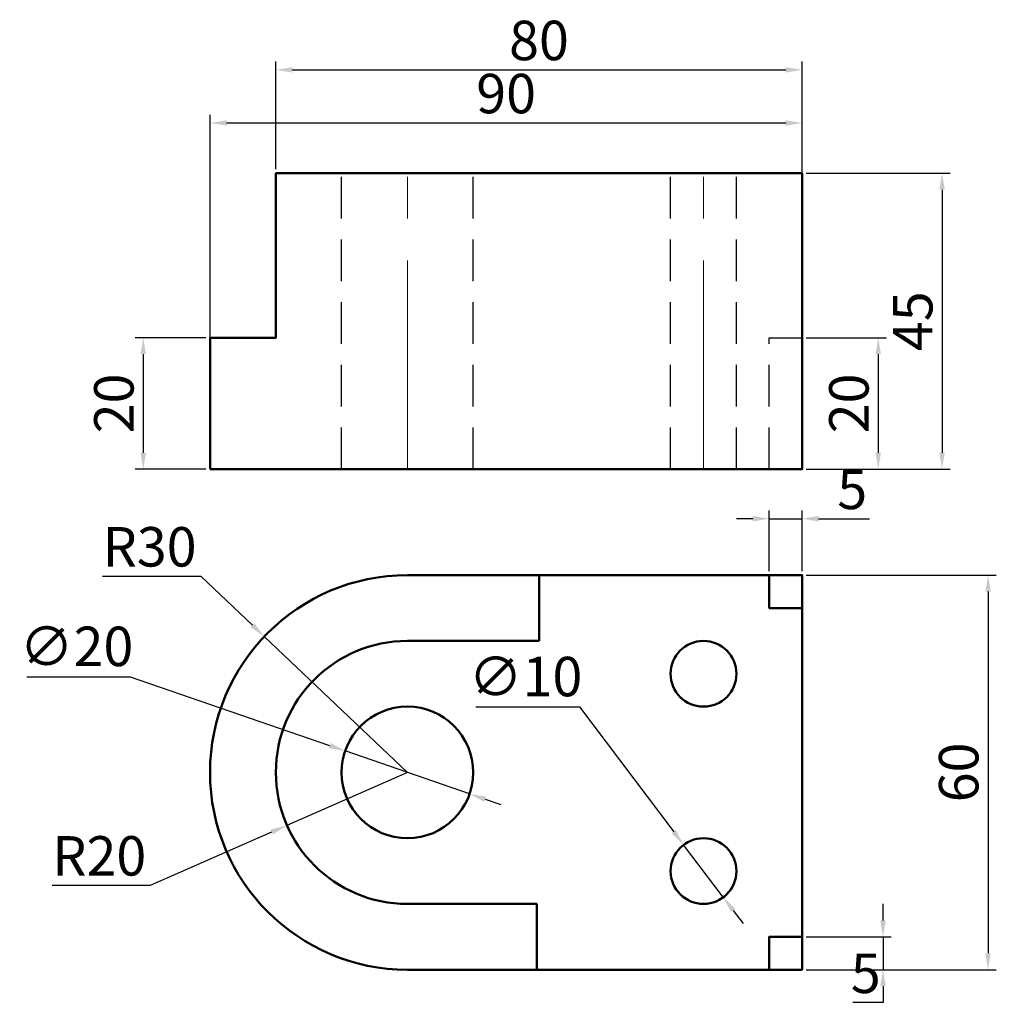
# Model space of a CAD drawing. Units: millimetres. Extents: x 12 to 160, y 72 to 221.
import ezdxf

# ---------------------------------------------------------------- set-up
doc = ezdxf.new("R2010")
doc.units = ezdxf.units.MM
doc.linetypes.add('CENTER', pattern=[50.8, 31.75, -6.35, 6.35, -6.35])
doc.linetypes.add('HIDDEN', pattern=[9.525, 6.35, -3.175])
for name, color, linetype, lineweight in [('M-CNTR', 1, 'CENTER', 18), ('M-DIMS', 2, 'Continuous', 25), ('M-HIDN', 4, 'HIDDEN', 25), ('M-OUTL', 7, 'Continuous', 50)]:
    doc.layers.add(name, color=color, linetype=linetype, lineweight=lineweight)
doc.styles.get("Standard").update_dxf_attribs({"font": 'arial.ttf'})
doc.dimstyles.new('ISO-25', dxfattribs={"dimtxt": 6, "dimasz": 2.5, "dimexe": 1.25, "dimexo": 0.625, "dimtad": 1, "dimtoh": 1, "dimdec": 0, "dimtxsty": 'Standard', "dimcen": 2.5, "dimadec": 0, "dimazin": 0, "dimtfac": 1, "dimtdec": 0, "dimtmove": 0, "dimatfit": 3, "dimfxl": 1, "dimarcsym": 0})

# ---------------------------------------------------------------- blocks, each defined once
blk = doc.blocks.new('*D1')
at = {"layer": 'Defpoints', "color": 0, "transparency": 16777216}
for p in [(130.64, 213.64), (50.64, 197.91), (130.64, 197.91)]:
    blk.add_point(p, dxfattribs=at)
at = {"layer": 'M-DIMS', "color": 0, "lineweight": -2, "transparency": 16777216}
for p, q in [((50.64, 198.53), (50.64, 214.89)), ((130.64, 198.53), (130.64, 214.89)), ((53.14, 213.64), (128.14, 213.64))]:
    blk.add_line(p, q, dxfattribs=at)
at = {"layer": 'M-DIMS', "color": 0, "transparency": 16777216}
for points in [[(53.14, 214.05), (53.14, 213.22), (50.64, 213.64)], [(128.14, 214.05), (128.14, 213.22), (130.64, 213.64)]]:
    blk.add_solid(points, dxfattribs=at)
at = {"layer": 'M-DIMS', "color": 0, "transparency": 16777216, "insert": (90.64, 217.33), "char_height": 6, "attachment_point": 5}
blk.add_mtext('80', dxfattribs=at)
blk = doc.blocks.new('*D2')
at = {"layer": 'Defpoints', "color": 0, "transparency": 16777216}
for p in [(130.64, 197.91), (130.64, 152.91), (151.9, 152.91)]:
    blk.add_point(p, dxfattribs=at)
at = {"layer": 'M-DIMS', "color": 0, "lineweight": -2, "transparency": 16777216}
for p, q in [((131.26, 197.91), (153.15, 197.91)), ((151.9, 195.41), (151.9, 155.41)), ((131.26, 152.91), (153.15, 152.91))]:
    blk.add_line(p, q, dxfattribs=at)
at = {"layer": 'M-DIMS', "color": 0, "transparency": 16777216}
for points in [[(151.48, 195.41), (152.32, 195.41), (151.9, 197.91)], [(151.48, 155.41), (152.32, 155.41), (151.9, 152.91)]]:
    blk.add_solid(points, dxfattribs=at)
at = {"layer": 'M-DIMS', "color": 0, "transparency": 16777216, "insert": (148.22, 175.41), "char_height": 6, "attachment_point": 5, "rotation": 90}
blk.add_mtext('45', dxfattribs=at)
blk = doc.blocks.new('*D3')
at = {"layer": 'Defpoints', "color": 0, "transparency": 16777216}
for p in [(40.64, 172.91), (30.49, 152.91), (40.64, 152.91)]:
    blk.add_point(p, dxfattribs=at)
at = {"layer": 'M-DIMS', "color": 0, "lineweight": -2, "transparency": 16777216}
for p, q in [((40.01, 172.91), (29.24, 172.91)), ((30.49, 170.41), (30.49, 155.41)), ((40.01, 152.91), (29.24, 152.91))]:
    blk.add_line(p, q, dxfattribs=at)
at = {"layer": 'M-DIMS', "color": 0, "transparency": 16777216}
for points in [[(30.07, 170.41), (30.9, 170.41), (30.49, 172.91)], [(30.07, 155.41), (30.9, 155.41), (30.49, 152.91)]]:
    blk.add_solid(points, dxfattribs=at)
at = {"layer": 'M-DIMS', "color": 0, "transparency": 16777216, "insert": (26.8, 162.91), "char_height": 6, "attachment_point": 5, "rotation": 90}
blk.add_mtext('20', dxfattribs=at)
blk = doc.blocks.new('*D4')
at = {"layer": 'Defpoints', "color": 0, "transparency": 16777216}
for p in [(130.64, 172.91), (130.64, 152.91), (142.21, 152.91)]:
    blk.add_point(p, dxfattribs=at)
at = {"layer": 'M-DIMS', "color": 0, "lineweight": -2, "transparency": 16777216}
for p, q in [((131.26, 172.91), (143.46, 172.91)), ((142.21, 170.41), (142.21, 155.41)), ((131.26, 152.91), (143.46, 152.91))]:
    blk.add_line(p, q, dxfattribs=at)
at = {"layer": 'M-DIMS', "color": 0, "transparency": 16777216}
for points in [[(141.79, 170.41), (142.62, 170.41), (142.21, 172.91)], [(141.79, 155.41), (142.62, 155.41), (142.21, 152.91)]]:
    blk.add_solid(points, dxfattribs=at)
at = {"layer": 'M-DIMS', "color": 0, "transparency": 16777216, "insert": (138.52, 162.91), "char_height": 6, "attachment_point": 5, "rotation": 90}
blk.add_mtext('20', dxfattribs=at)
blk = doc.blocks.new('*D5')
at = {"layer": 'Defpoints', "color": 0, "transparency": 16777216}
for p in [(130.64, 145.38), (125.64, 136.8), (130.64, 136.8)]:
    blk.add_point(p, dxfattribs=at)
at = {"layer": 'M-DIMS', "color": 0, "lineweight": -2, "transparency": 16777216}
for p, q in [((123.14, 145.38), (120.64, 145.38)), ((125.64, 137.42), (125.64, 146.63)), ((125.64, 145.38), (130.64, 145.38)), ((130.64, 137.42), (130.64, 146.63)), ((133.14, 145.38), (140.87, 145.38))]:
    blk.add_line(p, q, dxfattribs=at)
at = {"layer": 'M-DIMS', "color": 0, "transparency": 16777216}
for points in [[(123.14, 145.8), (123.14, 144.96), (125.64, 145.38)], [(133.14, 145.8), (133.14, 144.96), (130.64, 145.38)]]:
    blk.add_solid(points, dxfattribs=at)
at = {"layer": 'M-DIMS', "color": 0, "transparency": 16777216, "insert": (138.25, 149.06), "char_height": 6, "attachment_point": 5}
blk.add_mtext('5', dxfattribs=at)
blk = doc.blocks.new('*D6')
at = {"layer": 'Defpoints', "color": 0, "transparency": 16777216}
for p in [(130.64, 81.8), (130.64, 76.8), (142.93, 76.8)]:
    blk.add_point(p, dxfattribs=at)
at = {"layer": 'M-DIMS', "color": 0, "lineweight": -2, "transparency": 16777216}
for p, q in [((142.93, 84.3), (142.93, 86.8)), ((131.26, 81.8), (144.18, 81.8)), ((142.93, 81.8), (142.93, 76.8)), ((131.26, 76.8), (144.18, 76.8)), ((142.93, 74.3), (142.93, 71.8)), ((142.93, 71.8), (138.33, 71.8))]:
    blk.add_line(p, q, dxfattribs=at)
at = {"layer": 'M-DIMS', "color": 0, "transparency": 16777216}
for points in [[(142.51, 84.3), (143.35, 84.3), (142.93, 81.8)], [(142.51, 74.3), (143.35, 74.3), (142.93, 76.8)]]:
    blk.add_solid(points, dxfattribs=at)
at = {"layer": 'M-DIMS', "color": 0, "transparency": 16777216, "insert": (140.31, 75.47), "char_height": 6, "attachment_point": 5}
blk.add_mtext('5', dxfattribs=at)
blk = doc.blocks.new('*D7')
at = {"layer": 'Defpoints', "color": 0, "transparency": 16777216}
for p in [(130.64, 136.8), (130.64, 76.8), (158.9, 76.8)]:
    blk.add_point(p, dxfattribs=at)
at = {"layer": 'M-DIMS', "color": 0, "lineweight": -2, "transparency": 16777216}
for p, q in [((131.26, 136.8), (160.15, 136.8)), ((158.9, 134.3), (158.9, 79.3)), ((131.26, 76.8), (160.15, 76.8))]:
    blk.add_line(p, q, dxfattribs=at)
at = {"layer": 'M-DIMS', "color": 0, "transparency": 16777216}
for points in [[(158.48, 134.3), (159.31, 134.3), (158.9, 136.8)], [(158.48, 79.3), (159.31, 79.3), (158.9, 76.8)]]:
    blk.add_solid(points, dxfattribs=at)
at = {"layer": 'M-DIMS', "color": 0, "transparency": 16777216, "insert": (155.21, 106.8), "char_height": 6, "attachment_point": 5, "rotation": 90}
blk.add_mtext('60', dxfattribs=at)
blk = doc.blocks.new('*D8')
at = {"layer": 'Defpoints', "color": 0, "transparency": 16777216}
for p in [(48.89, 127.46), (70.64, 106.8)]:
    blk.add_point(p, dxfattribs=at)
at = {"layer": 'M-DIMS', "color": 0, "lineweight": -2, "transparency": 16777216}
for p, q in [((24.3, 136.64), (39.24, 136.64)), ((39.24, 136.64), (47.08, 129.19)), ((70.64, 106.8), (48.89, 127.46))]:
    blk.add_line(p, q, dxfattribs=at)
at = {"layer": 'M-DIMS', "color": 0, "transparency": 16777216}
blk.add_solid([(47.37, 129.49), (46.79, 128.88), (48.89, 127.46)], dxfattribs=at)
at = {"layer": 'M-DIMS', "color": 0, "transparency": 16777216, "insert": (31.45, 140.33), "char_height": 6, "attachment_point": 5}
blk.add_mtext('R30', dxfattribs=at)
blk = doc.blocks.new('*D9')
at = {"layer": 'Defpoints', "color": 0, "transparency": 16777216}
for p in [(70.64, 106.8), (52.33, 98.75)]:
    blk.add_point(p, dxfattribs=at)
at = {"layer": 'M-DIMS', "color": 0, "lineweight": -2, "transparency": 16777216}
for p, q in [((70.64, 106.8), (52.33, 98.75)), ((31.58, 89.64), (50.04, 97.75)), ((16.64, 89.64), (31.58, 89.64))]:
    blk.add_line(p, q, dxfattribs=at)
at = {"layer": 'M-DIMS', "color": 0, "transparency": 16777216}
blk.add_solid([(49.87, 98.13), (50.21, 97.37), (52.33, 98.75)], dxfattribs=at)
at = {"layer": 'M-DIMS', "color": 0, "transparency": 16777216, "insert": (23.8, 93.33), "char_height": 6, "attachment_point": 5}
blk.add_mtext('R20', dxfattribs=at)
blk = doc.blocks.new('*D10')
at = {"layer": 'Defpoints', "color": 0, "transparency": 16777216}
for p in [(61.19, 110.06), (80.09, 103.53)]:
    blk.add_point(p, dxfattribs=at)
at = {"layer": 'M-DIMS', "color": 0, "lineweight": -2, "transparency": 16777216}
for p, q in [((12.79, 121.34), (28.52, 121.34)), ((28.52, 121.34), (58.82, 110.88)), ((80.09, 103.53), (61.19, 110.06)), ((82.45, 102.72), (84.82, 101.9))]:
    blk.add_line(p, q, dxfattribs=at)
at = {"layer": 'M-DIMS', "color": 0, "transparency": 16777216}
for points in [[(58.96, 111.27), (58.69, 110.48), (61.19, 110.06)], [(82.59, 103.11), (82.32, 102.32), (80.09, 103.53)]]:
    blk.add_solid(points, dxfattribs=at)
at = {"layer": 'M-DIMS', "color": 0, "transparency": 16777216, "insert": (20.34, 125.19), "char_height": 6, "attachment_point": 5}
blk.add_mtext('∅20', dxfattribs=at)
blk = doc.blocks.new('*D11')
at = {"layer": 'Defpoints', "color": 0, "transparency": 16777216}
for p in [(112.62, 95.79), (118.65, 87.81)]:
    blk.add_point(p, dxfattribs=at)
at = {"layer": 'M-DIMS', "color": 0, "lineweight": -2, "transparency": 16777216}
for p, q in [((81.04, 116.75), (96.77, 116.75)), ((96.77, 116.75), (111.12, 97.78)), ((118.65, 87.81), (112.62, 95.79)), ((120.16, 85.82), (121.67, 83.82))]:
    blk.add_line(p, q, dxfattribs=at)
at = {"layer": 'M-DIMS', "color": 0, "transparency": 16777216}
for points in [[(111.45, 98.03), (110.78, 97.53), (112.62, 95.79)], [(120.5, 86.07), (119.83, 85.56), (118.65, 87.81)]]:
    blk.add_solid(points, dxfattribs=at)
at = {"layer": 'M-DIMS', "color": 0, "transparency": 16777216, "insert": (88.59, 120.6), "char_height": 6, "attachment_point": 5}
blk.add_mtext('∅10', dxfattribs=at)
blk = doc.blocks.new('*D12')
at = {"layer": 'Defpoints', "color": 0, "transparency": 16777216}
for p in [(130.64, 205.56), (40.64, 152.91), (130.64, 152.91)]:
    blk.add_point(p, dxfattribs=at)
at = {"layer": 'M-DIMS', "color": 0, "lineweight": -2, "transparency": 16777216}
for p, q in [((40.64, 153.53), (40.64, 206.81)), ((130.64, 153.53), (130.64, 206.81)), ((43.14, 205.56), (128.14, 205.56))]:
    blk.add_line(p, q, dxfattribs=at)
at = {"layer": 'M-DIMS', "color": 0, "transparency": 16777216}
for points in [[(43.14, 205.97), (43.14, 205.14), (40.64, 205.56)], [(128.14, 205.97), (128.14, 205.14), (130.64, 205.56)]]:
    blk.add_solid(points, dxfattribs=at)
at = {"layer": 'M-DIMS', "color": 0, "transparency": 16777216, "insert": (85.64, 209.25), "char_height": 6, "attachment_point": 5}
blk.add_mtext('90', dxfattribs=at)

msp = doc.modelspace()

# ---------------------------------------------------------------- linework, layer by layer
at = {"layer": 'M-CNTR'}
for p, q in [((70.64, 152.91), (70.64, 197.91)), ((115.64, 152.91), (115.64, 197.91))]:
    msp.add_line(p, q, dxfattribs=at)
at = {"layer": 'M-HIDN'}
for p, q in [((60.64, 152.91), (60.64, 197.91)), ((80.64, 152.91), (80.64, 197.91)), ((110.64, 152.91), (110.64, 197.91)), ((120.64, 152.91), (120.64, 197.91))]:
    msp.add_line(p, q, dxfattribs=at)
msp.add_lwpolyline([(125.64, 152.91), (125.64, 172.91), (130.64, 172.91)], dxfattribs=at)
at = {"layer": 'M-OUTL'}
for p, q in [((90.64, 126.8), (90.64, 136.8)), ((90.32, 86.8), (90.32, 76.8))]:
    msp.add_line(p, q, dxfattribs=at)
msp.add_lwpolyline([(40.64, 152.91), (40.64, 172.91), (50.64, 172.91), (50.64, 197.91), (130.64, 197.91), (130.64, 152.91)], close=True, dxfattribs=at)
msp.add_lwpolyline([(70.64, 136.8), (130.64, 136.8), (130.64, 76.8), (70.64, 76.8, -1)], format="xyb", close=True, dxfattribs=at)
for points in [[(125.64, 136.8), (125.64, 131.8), (130.64, 131.8)], [(125.64, 76.8), (125.64, 81.8), (130.64, 81.8)]]:
    msp.add_lwpolyline(points, dxfattribs=at)
msp.add_lwpolyline([(90.64, 126.8), (70.64, 126.8, 1), (70.64, 86.8), (90.32, 86.8)], format="xyb", dxfattribs=at)
for centre, radius in [((115.64, 121.8), 5), ((70.64, 106.8), 10), ((115.64, 91.8), 5)]:
    msp.add_circle(centre, radius, dxfattribs=at)

# ---------------------------------------------------------------- dimensions: what is measured, and where the dimension line sits
at = {"layer": 'M-DIMS'}
for base, p1, p2, override, picture, middle in [((130.64, 213.64), (50.64, 197.91), (130.64, 197.91), {"dimclrd": 0, "dimclre": 0, "dimclrt": 0}, '*D1', (90.64, 217.33)), ((130.64, 205.56), (40.64, 152.91), (130.64, 152.91), {"dimdec": 0, "dimlfac": 1, "dimrnd": 0, "dimzin": 0, "dimdsep": 46, "dimlunit": 2}, '*D12', (85.64, 209.25)), ((130.64, 145.38), (125.64, 136.8), (130.64, 136.8), {"dimclrd": 0, "dimclre": 0, "dimclrt": 0}, '*D5', (138.25, 149.06))]:
    dim = msp.add_linear_dim(base=base, p1=p1, p2=p2, dimstyle='ISO-25', override=override, dxfattribs=at)
    dim.commit()
    dim.dimension.update_dxf_attribs({"geometry": picture, "text_midpoint": middle})
for base, p1, p2, picture, middle in [((151.9, 152.91), (130.64, 197.91), (130.64, 152.91), '*D2', (148.22, 175.41)), ((30.49, 152.91), (40.64, 172.91), (40.64, 152.91), '*D3', (26.8, 162.91)), ((142.21, 152.91), (130.64, 172.91), (130.64, 152.91), '*D4', (138.52, 162.91)), ((158.9, 76.8), (130.64, 136.8), (130.64, 76.8), '*D7', (155.21, 106.8)), ((142.93, 76.8), (130.64, 81.8), (130.64, 76.8), '*D6', (140.31, 75.47))]:
    dim = msp.add_linear_dim(base=base, p1=p1, p2=p2, angle=90, dimstyle='ISO-25', override={"dimclrd": 0, "dimclre": 0, "dimclrt": 0}, dxfattribs=at)
    dim.commit()
    dim.dimension.update_dxf_attribs({"geometry": picture, "text_midpoint": middle})
for mpoint, picture, middle in [((48.89, 127.46), '*D8', (31.45, 136.64)), ((52.33, 98.75), '*D9', (23.8, 89.64))]:
    dim = msp.add_radius_dim(center=(70.64, 106.8), mpoint=mpoint, dimstyle='ISO-25', override={"dimclrd": 0, "dimclre": 0, "dimclrt": 0}, dxfattribs=at)
    dim.commit()
    dim.dimension.update_dxf_attribs({"geometry": picture, "text_midpoint": middle, "dimtype": 164})
for p1, p2, picture, middle in [((80.09, 103.53), (61.19, 110.06), '*D10', (20.34, 121.34)), ((118.65, 87.81), (112.62, 95.79), '*D11', (88.59, 116.75))]:
    dim = msp.add_diameter_dim_2p(p1=p1, p2=p2, dimstyle='ISO-25', override={"dimclrd": 0, "dimclre": 0, "dimclrt": 0}, dxfattribs=at)
    dim.commit()
    dim.dimension.update_dxf_attribs({"geometry": picture, "text_midpoint": middle, "dimtype": 163})

doc.saveas('drawing.dxf')
